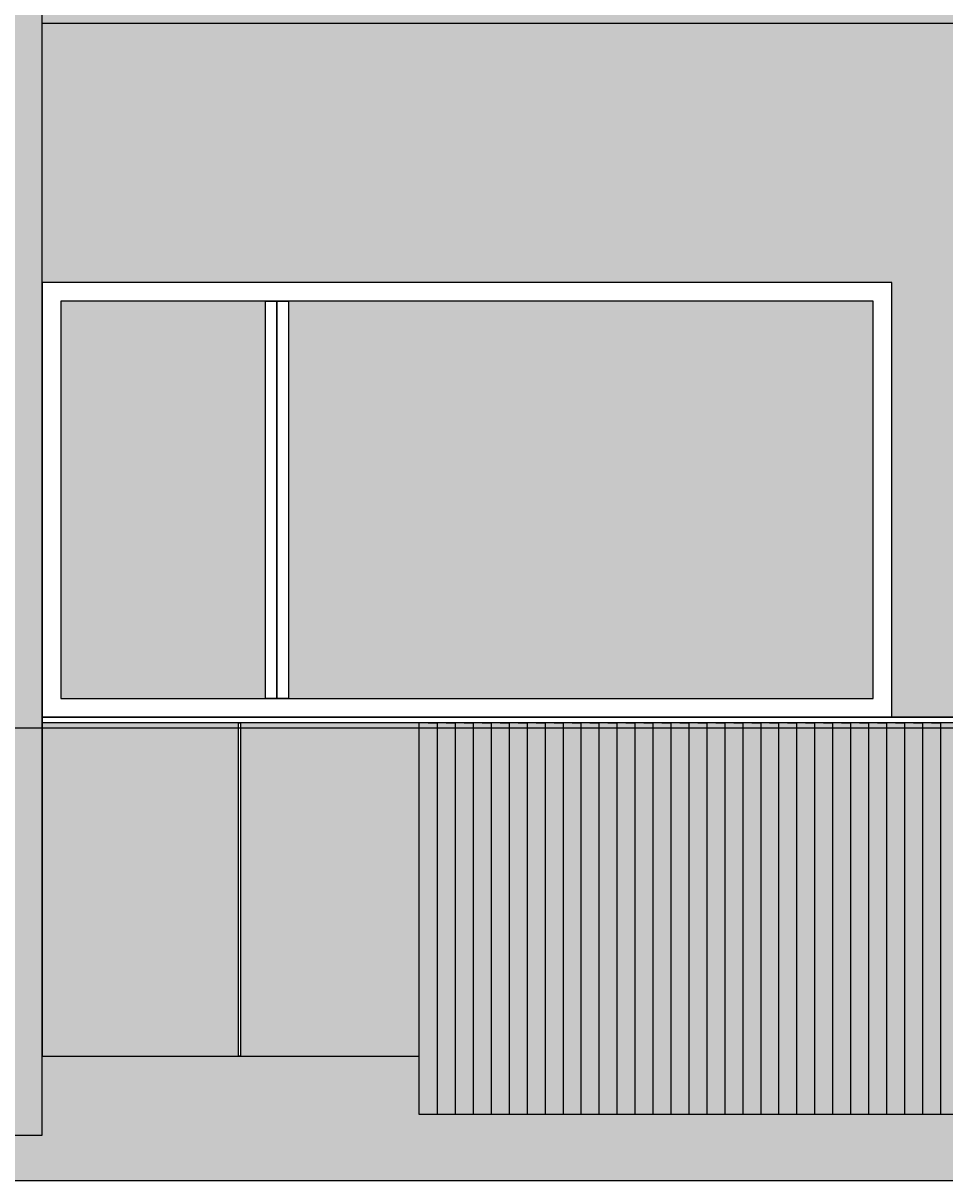
# Model space of a CAD drawing. Units: feet. Extents: x 2193 to 3502, y 890 to 1601.
# Tile 4 of 17: x 2466 to 2587, y 1073 to 1225. Entities that reach past the tile are written whole.
import ezdxf

# ---------------------------------------------------------------- set-up
doc = ezdxf.new("R2010")
doc.units = ezdxf.units.FT
for name, color, linetype, lineweight in [('A-ANNO-DIMS', 2, 'Continuous', 18), ('A-ELEV', 7, 'Continuous', 25), ('A-ELEV-PATT', 8, 'Continuous', 13)]:
    doc.layers.add(name, color=color, linetype=linetype, lineweight=lineweight)
doc.styles.get("Standard").update_dxf_attribs({"font": 'arial.ttf'})
doc.dimstyles.get("Standard").update_dxf_attribs({"dimtxt": 0.18, "dimasz": 0.18, "dimexe": 0.18, "dimexo": 0.0625, "dimgap": 0.09, "dimtad": 0, "dimtih": 1, "dimtoh": 1, "dimdec": 0, "dimzin": 0, "dimdsep": 46, "dimlunit": 3, "dimtxsty": 'Standard', "dimcen": 0.09, "dimadec": 0, "dimazin": 0, "dimtfac": 1, "dimtdec": 0, "dimtofl": 0, "dimtmove": 0, "dimatfit": 3, "dimfxl": 1, "dimtolj": 1, "dimtzin": 0, "dimarcsym": 0})

# ---------------------------------------------------------------- blocks, each defined once
blk = doc.blocks.new('*D19')
at = {"layer": 'A-ANNO-DIMS', "color": 0, "lineweight": -2, "transparency": 16777216}
for p, q in [((2934.31, 1073.03), (2193.56, 1073.03)), ((2193.74, 1072.85), (2193.74, 1012.11)), ((2193.74, 951), (2193.74, 1011.75)), ((2934.31, 950.82), (2193.56, 950.82))]:
    blk.add_line(p, q, dxfattribs=at)
at = {"layer": 'A-ANNO-DIMS', "color": 0, "transparency": 16777216}
for points in [[(2193.71, 1072.85), (2193.77, 1072.85), (2193.74, 1073.03)], [(2193.71, 951), (2193.77, 951), (2193.74, 950.82)]]:
    blk.add_solid(points, dxfattribs=at)
at = {"layer": 'Defpoints', "color": 0, "transparency": 16777216}
for p in [(2193.74, 1073.03), (2934.37, 1073.03), (2934.37, 950.82)]:
    blk.add_point(p, dxfattribs=at)
at = {"layer": 'A-ANNO-DIMS', "color": 0, "transparency": 16777216, "insert": (2193.74, 1011.93), "char_height": 0.18, "attachment_point": 5}
blk.add_mtext('\\A1;122.2', dxfattribs=at)
blk = doc.blocks.new('*D20')
at = {"layer": 'A-ANNO-DIMS', "color": 0, "lineweight": -2, "transparency": 16777216}
for p, q in [((2933.15, 1408.48), (2193.56, 1408.48)), ((2193.74, 1408.3), (2193.74, 1240.94)), ((2193.74, 1073.21), (2193.74, 1240.57)), ((2934.31, 1073.03), (2193.56, 1073.03))]:
    blk.add_line(p, q, dxfattribs=at)
at = {"layer": 'A-ANNO-DIMS', "color": 0, "transparency": 16777216}
for points in [[(2193.71, 1408.3), (2193.77, 1408.3), (2193.74, 1408.48)], [(2193.71, 1073.21), (2193.77, 1073.21), (2193.74, 1073.03)]]:
    blk.add_solid(points, dxfattribs=at)
at = {"layer": 'Defpoints', "color": 0, "transparency": 16777216}
for p in [(2193.74, 1408.48), (2933.21, 1408.48), (2934.37, 1073.03)]:
    blk.add_point(p, dxfattribs=at)
at = {"layer": 'A-ANNO-DIMS', "color": 0, "transparency": 16777216, "insert": (2193.74, 1240.76), "char_height": 0.18, "attachment_point": 5}
blk.add_mtext('\\A1;335.45', dxfattribs=at)
blk = doc.blocks.new('*D26')
at = {"layer": 'A-ANNO-DIMS', "color": 0, "lineweight": -2, "transparency": 16777216}
for p, q in [((2255.16, 950.89), (2255.16, 1601.47)), ((2255.34, 1601.29), (2507.42, 1601.29)), ((2760.29, 1601.29), (2508.21, 1601.29)), ((2760.47, 1541.11), (2760.47, 1601.47))]:
    blk.add_line(p, q, dxfattribs=at)
at = {"layer": 'A-ANNO-DIMS', "color": 0, "transparency": 16777216}
for points in [[(2255.34, 1601.32), (2255.34, 1601.26), (2255.16, 1601.29)], [(2760.29, 1601.32), (2760.29, 1601.26), (2760.47, 1601.29)]]:
    blk.add_solid(points, dxfattribs=at)
at = {"layer": 'Defpoints', "color": 0, "transparency": 16777216}
for p in [(2760.47, 1601.29), (2760.47, 1541.04), (2255.16, 950.82)]:
    blk.add_point(p, dxfattribs=at)
at = {"layer": 'A-ANNO-DIMS', "color": 0, "transparency": 16777216, "insert": (2507.82, 1601.29), "char_height": 0.18, "attachment_point": 5}
blk.add_mtext('\\A1;505.3', dxfattribs=at)
blk = doc.blocks.new('*D35')
at = {"layer": 'A-ANNO-DIMS', "color": 0, "lineweight": -2, "transparency": 16777216}
for p, q in [((2980.65, 1132.39), (2193.56, 1132.39)), ((2193.74, 1132.21), (2193.74, 1102.89)), ((2193.74, 1073.21), (2193.74, 1102.53)), ((2934.31, 1073.03), (2193.56, 1073.03))]:
    blk.add_line(p, q, dxfattribs=at)
at = {"layer": 'A-ANNO-DIMS', "color": 0, "transparency": 16777216}
for points in [[(2193.71, 1132.21), (2193.77, 1132.21), (2193.74, 1132.39)], [(2193.71, 1073.21), (2193.77, 1073.21), (2193.74, 1073.03)]]:
    blk.add_solid(points, dxfattribs=at)
at = {"layer": 'Defpoints', "color": 0, "transparency": 16777216}
for p in [(2193.74, 1132.39), (2980.72, 1132.39), (2934.37, 1073.03)]:
    blk.add_point(p, dxfattribs=at)
at = {"layer": 'A-ANNO-DIMS', "color": 0, "transparency": 16777216, "insert": (2193.74, 1102.71), "char_height": 0.18, "attachment_point": 5}
blk.add_mtext('\\A1;59.36', dxfattribs=at)
blk = doc.blocks.new('*D36')
at = {"layer": 'A-ANNO-DIMS', "color": 0, "lineweight": -2, "transparency": 16777216}
for p, q in [((2974.05, 1268.66), (2193.56, 1268.66)), ((2193.74, 1268.48), (2193.74, 1200.71)), ((2193.74, 1132.57), (2193.74, 1200.34)), ((2980.65, 1132.39), (2193.56, 1132.39))]:
    blk.add_line(p, q, dxfattribs=at)
at = {"layer": 'A-ANNO-DIMS', "color": 0, "transparency": 16777216}
for points in [[(2193.71, 1268.48), (2193.77, 1268.48), (2193.74, 1268.66)], [(2193.71, 1132.57), (2193.77, 1132.57), (2193.74, 1132.39)]]:
    blk.add_solid(points, dxfattribs=at)
at = {"layer": 'Defpoints', "color": 0, "transparency": 16777216}
for p in [(2193.74, 1268.66), (2974.12, 1268.66), (2980.72, 1132.39)]:
    blk.add_point(p, dxfattribs=at)
at = {"layer": 'A-ANNO-DIMS', "color": 0, "transparency": 16777216, "insert": (2193.74, 1200.53), "char_height": 0.18, "attachment_point": 5}
blk.add_mtext('\\A1;136.27', dxfattribs=at)

msp = doc.modelspace()

# ---------------------------------------------------------------- hatches: boundary and pattern name
at = {"layer": 'A-ELEV-PATT'}
h = msp.add_hatch(color=256, dxfattribs=at)
h.dxf.hatch_style = 1
h.paths.add_polyline_path([(2760.4733, 1512.3957), (2586.1736, 1512.3957), (2586.1736, 1502.0763), (2602.8648, 1502.0763), (2699.5726, 1502.0763), (2699.6322, 1502.0763), (2760.4733, 1502.0763)])
h.paths.add_polyline_path([(2760.4733, 1382.0763), (2275.0482, 1382.0763), (2275.0482, 1367.5739), (2745.971, 1367.5739), (2745.971, 1166.2327), (2760.4733, 1166.2327)])
h.paths.add_polyline_path([(2468.2854, 1266.7092), (2294.8992, 1266.7092), (2294.8992, 1079.031), (2468.2854, 1079.031)])
h.paths.add_polyline_path([(2301.4984, 1260.11), (2461.6863, 1260.11), (2461.6863, 1085.6301), (2301.4984, 1085.6301)], flags=16)
h.paths.add_polyline_path([(2452.7821, 1241.1967), (2452.7821, 1217.2819), (2454.6216, 1217.2819), (2454.6216, 1133.1367), (2461.6863, 1133.1367), (2461.6863, 1132.3937), (2381.7172, 1132.3937), (2381.7172, 1085.6301), (2381.4675, 1085.6301), (2381.4675, 1132.3937), (2301.4984, 1132.3937), (2301.4984, 1133.1367), (2301.4984, 1217.2819), (2390.8933, 1217.2819), (2390.8933, 1241.1967)], flags=0)
h.paths.add_polyline_path([(2372.4936, 1214.8367), (2372.4936, 1133.1367), (2371.1246, 1133.1367), (2371.1246, 1214.8367), (2337.2323, 1214.8367), (2337.2323, 1133.1367), (2335.8632, 1133.1367), (2335.8632, 1214.8367), (2337.2323, 1214.8367)], flags=0)
h = msp.add_hatch(color=256, dxfattribs=at)
h.dxf.hatch_style = 1
h.paths.add_polyline_path([(2576.3428, 1407.7384), (2536.5416, 1407.7384), (2536.5416, 1406.15), (2536.5416, 1382.0763), (2576.3428, 1382.0763)])
h.paths.add_polyline_path([(2627.3548, 1407.7384), (2576.5924, 1407.7384), (2576.5924, 1382.0763), (2627.3548, 1382.0763)])
h.paths.add_polyline_path([(2667.9236, 1407.7384), (2627.6045, 1407.7384), (2627.6045, 1382.0763), (2667.9236, 1382.0763)])
h.paths.add_polyline_path([(2699.6322, 1407.7384), (2668.1733, 1407.7384), (2668.1733, 1382.0763), (2699.6322, 1382.0763)])
h.paths.add_polyline_path([(2497.5717, 1323.2248), (2470.7305, 1323.2248), (2470.7305, 1271.105), (2497.5717, 1271.105)])
h.paths.add_polyline_path([(2577.3219, 1323.2248), (2500.599, 1323.2248), (2500.599, 1271.105), (2577.3219, 1271.105)])
h.paths.add_polyline_path([(2388.4482, 1327.1314), (2343.4244, 1327.1314), (2343.4244, 1268.6599), (2388.4482, 1268.6599)])
h.paths.add_polyline_path([(2342.3682, 1327.1314), (2297.3443, 1327.1314), (2297.3443, 1268.6599), (2342.3682, 1268.6599)])
h.paths.add_polyline_path([(2335.8632, 1214.8367), (2301.4984, 1214.8367), (2301.4984, 1133.1367), (2335.8632, 1133.1367)])
h.paths.add_polyline_path([(2371.1246, 1214.8367), (2337.2323, 1214.8367), (2337.2323, 1133.1367), (2371.1246, 1133.1367)])
h.paths.add_polyline_path([(2390.8933, 1214.8367), (2372.4936, 1214.8367), (2372.4936, 1133.1367), (2390.8933, 1133.1367)])
h.paths.add_polyline_path([(2577.3219, 1188.4208), (2500.599, 1188.4208), (2500.599, 1136.3009), (2577.3219, 1136.3009)])
h.paths.add_polyline_path([(2497.5717, 1188.4208), (2470.7305, 1188.4208), (2470.7305, 1136.3009), (2497.5717, 1136.3009)])
h.paths.add_polyline_path([(2381.4675, 1132.3937), (2301.4984, 1132.3937), (2301.4984, 1085.6301), (2381.4675, 1085.6301)])
h.paths.add_polyline_path([(2461.6863, 1132.3937), (2381.7172, 1132.3937), (2381.7172, 1085.6301), (2461.6863, 1085.6301)])
h.paths.add_polyline_path([(2494.0463, 1133.1128), (2468.2854, 1133.1128), (2468.2854, 1089.3627), (2494.0463, 1089.3627)])
h.paths.add_polyline_path([(2517.7591, 1133.1128), (2494.296, 1133.1128), (2494.296, 1089.3627), (2517.7591, 1089.3627)])
h.paths.add_polyline_path([(2667.9236, 1133.1128), (2636.5184, 1133.1128), (2636.5184, 1089.3627), (2667.9236, 1089.3627)])
h.paths.add_polyline_path([(2699.6322, 1133.1128), (2668.1733, 1133.1128), (2668.1733, 1089.3627), (2699.6322, 1089.3627)])
h.paths.add_polyline_path([(2651.839, 1070.5859), (2638.7977, 1070.5859), (2638.7977, 1047.0961), (2651.839, 1047.0961)])
h.paths.add_polyline_path([(2637.6317, 1070.5859), (2625.7563, 1070.5859), (2625.7563, 1047.0961), (2637.6317, 1047.0961)])
h.paths.add_polyline_path([(2583.4393, 1052.8618), (2515.9216, 1052.8618), (2515.9216, 1032.1935), (2583.4393, 1032.1935)])
h.paths.add_polyline_path([(2514.4293, 1052.8618), (2492.062, 1052.8618), (2492.062, 1032.1935), (2514.4293, 1032.1935)])
h.paths.add_polyline_path([(2388.4482, 1038.8658), (2348.7682, 1038.8658), (2348.7682, 988.9597), (2388.4482, 988.9597)])
h.paths.add_polyline_path([(2346.3231, 1038.8658), (2309.0883, 1038.8658), (2309.0883, 988.9597), (2346.3231, 988.9597)])
h.paths.add_polyline_path([(2667.9236, 1267.9169), (2636.5184, 1267.9169), (2636.5184, 1241.1967), (2667.9236, 1241.1967)])
h.paths.add_polyline_path([(2699.6322, 1267.9169), (2668.1733, 1267.9169), (2668.1733, 1241.1967), (2699.6322, 1241.1967)])
h.paths.add_polyline_path([(2517.7591, 1267.9169), (2494.296, 1267.9169), (2494.296, 1241.1967), (2517.7591, 1241.1967)])
h.paths.add_polyline_path([(2494.0463, 1267.9169), (2468.2854, 1267.9169), (2468.2854, 1266.7092), (2468.2854, 1241.1967), (2494.0463, 1241.1967)])
h = msp.add_hatch(color=256, dxfattribs=at)
h.dxf.hatch_style = 1
h.paths.add_polyline_path([(2294.8992, 1367.5739), (2275.0482, 1367.5739), (2275.0482, 1382.0763), (2536.5416, 1382.0763), (2536.5416, 1406.15), (2256.3232, 1406.15), (2256.3232, 1089.3627), (2255.1574, 1089.3627), (2255.1574, 1073.031), (2294.8992, 1073.031)])
h.paths.add_polyline_path([(2517.7591, 1241.1967), (2468.2854, 1241.1967), (2468.2854, 1224.865), (2598.591, 1224.865), (2598.591, 1233.561), (2517.7591, 1233.561)])
h.paths.add_polyline_path([(2699.6322, 1241.1967), (2636.5184, 1241.1967), (2636.5184, 1233.561), (2616.5596, 1233.561), (2616.5596, 1224.865), (2699.6322, 1224.865)])
h.paths.add_polyline_path([(2615.4622, 1233.561), (2613.8564, 1233.561), (2613.8564, 1224.865), (2615.4622, 1224.865)])
h.paths.add_polyline_path([(2612.759, 1233.561), (2609.5836, 1233.561), (2609.5836, 1224.865), (2612.759, 1224.865)])
h.paths.add_polyline_path([(2608.4862, 1233.561), (2606.5316, 1233.561), (2606.5316, 1224.865), (2608.4862, 1224.865)])
h.paths.add_polyline_path([(2605.4342, 1233.561), (2602.5204, 1233.561), (2602.5204, 1224.865), (2605.4342, 1224.865)])
h.paths.add_polyline_path([(2601.423, 1233.561), (2599.6883, 1233.561), (2599.6883, 1224.865), (2601.423, 1224.865)])
h.paths.add_polyline_path([(2517.7591, 1089.3627), (2468.2854, 1089.3627), (2468.2854, 1079.031), (2294.8992, 1079.031), (2294.8992, 1073.031), (2390.8933, 1073.031), (2452.7821, 1073.031), (2760.4733, 1073.031), (2760.4733, 1089.3627), (2699.6322, 1089.3627), (2636.5184, 1089.3627), (2636.5184, 1081.7269), (2517.7591, 1081.7269)])
h = msp.add_hatch(color=256, dxfattribs=at)
h.dxf.hatch_style = 1
h.paths.add_polyline_path([(2452.7821, 1355.2199), (2622.9814, 1355.2199), (2622.9814, 1268.6599), (2646.2844, 1268.6599), (2646.2844, 1367.5739), (2390.8933, 1367.5739), (2390.8933, 1268.6599), (2452.7821, 1268.6599)])
h.paths.add_polyline_path([(2452.7821, 1016.4), (2431.9134, 1016.4), (2431.9134, 1032.1935), (2452.7821, 1032.1935), (2452.7821, 1073.031), (2390.8933, 1073.031), (2390.8933, 956.8829), (2452.7821, 956.8829)])
h.paths.add_polyline_path([(2452.7821, 1241.1967), (2390.8933, 1241.1967), (2390.8933, 1133.1367), (2452.7821, 1133.1367)])
h.paths.add_polyline_path([(2636.5184, 1267.9169), (2517.7591, 1267.9169), (2517.7591, 1233.561), (2598.591, 1233.561), (2598.591, 1249.8256), (2599.6883, 1249.8256), (2599.6883, 1233.561), (2601.423, 1233.561), (2601.423, 1247.0422), (2602.5204, 1247.0422), (2602.5204, 1233.561), (2605.4342, 1233.561), (2605.4342, 1250.4403), (2606.5316, 1250.4403), (2606.5316, 1233.561), (2608.4862, 1233.561), (2608.4862, 1248.4363), (2609.5836, 1248.4363), (2609.5836, 1233.561), (2612.759, 1233.561), (2612.759, 1243.2956), (2613.8564, 1243.2956), (2613.8564, 1233.561), (2615.4622, 1233.561), (2615.4622, 1249.6561), (2616.5596, 1249.6561), (2616.5596, 1233.561), (2636.5184, 1233.561)])
h.paths.add_polyline_path([(2601.423, 1133.1128), (2599.6883, 1133.1128), (2599.6883, 1115.2331), (2598.591, 1115.2331), (2598.591, 1133.1128), (2517.7591, 1133.1128), (2517.7591, 1081.7269), (2636.5184, 1081.7269), (2636.5184, 1133.1128), (2616.5596, 1133.1128), (2616.5596, 1115.0637), (2615.4622, 1115.0637), (2615.4622, 1133.1128), (2613.8564, 1133.1128), (2613.8564, 1108.7032), (2612.759, 1108.7032), (2612.759, 1133.1128), (2609.5836, 1133.1128), (2609.5836, 1113.8439), (2608.4862, 1113.8439), (2608.4862, 1133.1128), (2606.5316, 1133.1128), (2606.5316, 1115.8479), (2605.4342, 1115.8479), (2605.4342, 1133.1128), (2602.5204, 1133.1128), (2602.5204, 1112.4498), (2601.423, 1112.4498)])
h = msp.add_hatch(color=256, dxfattribs=at)
h.dxf.hatch_style = 1
h.paths.add_polyline_path([(2622.9814, 1355.2199), (2452.7821, 1355.2199), (2452.7821, 1268.6599), (2468.2854, 1268.6599), (2468.2854, 1325.6699), (2579.767, 1325.6699), (2579.767, 1268.6599), (2622.9814, 1268.6599)])
h.paths.add_polyline_path([(2598.591, 1224.865), (2468.2854, 1224.865), (2468.2854, 1190.8659), (2579.767, 1190.8659), (2579.767, 1133.8558), (2598.591, 1133.8558)])
h.paths.add_polyline_path([(2390.8933, 1241.1967), (2301.4984, 1241.1967), (2301.4984, 1224.865), (2390.8933, 1224.865)])
h.paths.add_polyline_path([(3070.1101, 1073.031), (2940.0814, 1073.031), (2940.0814, 956.5285), (2940.6598, 956.8829), (3070.1101, 956.8829), (3070.1101, 986.5146), (2985.8599, 986.5146), (2985.8599, 1041.3109), (3070.1101, 1041.3109)])

# ---------------------------------------------------------------- linework, layer by layer
at = {"layer": 'A-ELEV'}
for p, q in [((2468.2854, 1224.865), (2699.6322, 1224.865)), ((2468.2854, 1089.3627), (2517.7591, 1089.3627)), ((2468.2854, 1089.3627), (2517.7591, 1089.3627))]:
    msp.add_line(p, q, dxfattribs=at)
for points in [[(2294.8992, 1079.031), (2468.2854, 1079.031), (2468.2854, 1266.7092), (2294.8992, 1266.7092)], [(2294.8992, 1079.031), (2468.2854, 1079.031), (2468.2854, 1266.7092), (2294.8992, 1266.7092)], [(2468.2854, 1133.8558), (2579.767, 1133.8558), (2579.767, 1190.8659), (2468.2854, 1190.8659)], [(2468.2854, 1133.8558), (2579.767, 1133.8558), (2579.767, 1190.8659), (2468.2854, 1190.8659)], [(2470.7305, 1136.3009), (2577.3219, 1136.3009), (2577.3219, 1188.4208), (2470.7305, 1188.4208)], [(2470.7305, 1136.3009), (2577.3219, 1136.3009), (2577.3219, 1188.4208), (2470.7305, 1188.4208)], [(2497.5717, 1188.4208), (2499.0853, 1188.4208), (2499.0853, 1136.3009), (2497.5717, 1136.3009)], [(2497.5717, 1188.4208), (2499.0853, 1188.4208), (2499.0853, 1136.3009), (2497.5717, 1136.3009)], [(2499.0853, 1188.4208), (2500.599, 1188.4208), (2500.599, 1136.3009), (2499.0853, 1136.3009)], [(2499.0853, 1188.4208), (2500.599, 1188.4208), (2500.599, 1136.3009), (2499.0853, 1136.3009)], [(2494.0463, 1133.1128), (2494.296, 1133.1128), (2494.296, 1089.3627), (2494.0463, 1089.3627)], [(2494.0463, 1133.1128), (2494.296, 1133.1128), (2494.296, 1089.3627), (2494.0463, 1089.3627)]]:
    msp.add_lwpolyline(points, close=True, dxfattribs=at)
for points in [[(2699.6322, 1133.8558), (2468.2854, 1133.8558), (2468.2854, 1089.3627)], [(2699.6322, 1133.1128), (2468.2854, 1133.1128), (2468.2854, 1133.8558), (2699.6322, 1133.8558)], [(2598.591, 1133.8558), (2468.2854, 1133.8558), (2468.2854, 1089.3627)], [(2598.591, 1133.1128), (2468.2854, 1133.1128), (2468.2854, 1133.8558), (2598.591, 1133.8558)], [(2636.5184, 1133.1128), (2636.5184, 1081.7269), (2517.7591, 1081.7269), (2517.7591, 1133.1128)], [(2636.5184, 1133.1128), (2636.5184, 1081.7269), (2517.7591, 1081.7269), (2517.7591, 1133.1128)], [(2518.938, 1133.1128), (2520.1169, 1133.1128), (2520.1169, 1081.7269), (2518.938, 1081.7269)], [(2521.2958, 1133.1128), (2522.4747, 1133.1128), (2522.4747, 1081.7269), (2521.2958, 1081.7269)], [(2523.6536, 1133.1128), (2524.8326, 1133.1128), (2524.8326, 1081.7269), (2523.6536, 1081.7269)], [(2526.0115, 1133.1128), (2527.1904, 1133.1128), (2527.1904, 1081.7269), (2526.0115, 1081.7269)], [(2528.3693, 1133.1128), (2529.5482, 1133.1128), (2529.5482, 1081.7269), (2528.3693, 1081.7269)], [(2530.7272, 1133.1128), (2531.9061, 1133.1128), (2531.9061, 1081.7269), (2530.7272, 1081.7269)], [(2533.085, 1133.1128), (2534.2639, 1133.1128), (2534.2639, 1081.7269), (2533.085, 1081.7269)], [(2535.4428, 1133.1128), (2536.6217, 1133.1128), (2536.6217, 1081.7269), (2535.4428, 1081.7269)], [(2537.8007, 1133.1128), (2538.9796, 1133.1128), (2538.9796, 1081.7269), (2537.8007, 1081.7269)], [(2540.1585, 1133.1128), (2541.3374, 1133.1128), (2541.3374, 1081.7269), (2540.1585, 1081.7269)], [(2542.5163, 1133.1128), (2543.6953, 1133.1128), (2543.6953, 1081.7269), (2542.5163, 1081.7269)], [(2544.8742, 1133.1128), (2546.0531, 1133.1128), (2546.0531, 1081.7269), (2544.8742, 1081.7269)], [(2547.232, 1133.1128), (2548.4109, 1133.1128), (2548.4109, 1081.7269), (2547.232, 1081.7269)], [(2549.5899, 1133.1128), (2550.7688, 1133.1128), (2550.7688, 1081.7269), (2549.5899, 1081.7269)], [(2551.9477, 1133.1128), (2553.1266, 1133.1128), (2553.1266, 1081.7269), (2551.9477, 1081.7269)], [(2554.3055, 1133.1128), (2555.4844, 1133.1128), (2555.4844, 1081.7269), (2554.3055, 1081.7269)], [(2556.6634, 1133.1128), (2557.8423, 1133.1128), (2557.8423, 1081.7269), (2556.6634, 1081.7269)], [(2559.0212, 1133.1128), (2560.2001, 1133.1128), (2560.2001, 1081.7269), (2559.0212, 1081.7269)], [(2561.379, 1133.1128), (2562.558, 1133.1128), (2562.558, 1081.7269), (2561.379, 1081.7269)], [(2563.7369, 1133.1128), (2564.9158, 1133.1128), (2564.9158, 1081.7269), (2563.7369, 1081.7269)], [(2566.0947, 1133.1128), (2567.2736, 1133.1128), (2567.2736, 1081.7269), (2566.0947, 1081.7269)], [(2568.4525, 1133.1128), (2569.6315, 1133.1128), (2569.6315, 1081.7269), (2568.4525, 1081.7269)], [(2570.8104, 1133.1128), (2571.9893, 1133.1128), (2571.9893, 1081.7269), (2570.8104, 1081.7269)], [(2573.1682, 1133.1128), (2574.3471, 1133.1128), (2574.3471, 1081.7269), (2573.1682, 1081.7269)], [(2575.5261, 1133.1128), (2576.705, 1133.1128), (2576.705, 1081.7269), (2575.5261, 1081.7269)], [(2577.8839, 1133.1128), (2579.0628, 1133.1128), (2579.0628, 1081.7269), (2577.8839, 1081.7269)], [(2580.2417, 1133.1128), (2581.4207, 1133.1128), (2581.4207, 1081.7269), (2580.2417, 1081.7269)], [(2582.5996, 1133.1128), (2583.7785, 1133.1128), (2583.7785, 1081.7269), (2582.5996, 1081.7269)], [(2584.9574, 1133.1128), (2586.1363, 1133.1128), (2586.1363, 1081.7269), (2584.9574, 1081.7269)]]:
    msp.add_lwpolyline(points, dxfattribs=at)

# ---------------------------------------------------------------- dimensions: what is measured, and where the dimension line sits
at = {"layer": 'A-ANNO-DIMS'}
dim = msp.add_linear_dim(base=(2760.4733, 1601.2941), p1=(2255.1574, 950.8228), p2=(2760.4733, 1541.0441), dimstyle='Standard', override={"dimdec": 1, "dimlfac": 1, "dimrnd": 0, "dimzin": 0, "dimdsep": 46, "dimlunit": 2}, dxfattribs=at)
dim.commit()
dim.dimension.update_dxf_attribs({"geometry": '*D26', "text_midpoint": (2507.8154, 1601.2941)})
for base, p1, p2, override, picture, middle in [((2193.7417, 1408.4814), (2934.3742, 1073.031), (2933.2085, 1408.4814), {"dimdec": 2, "dimlfac": 1, "dimrnd": 0, "dimzin": 0, "dimdsep": 46, "dimlunit": 2}, '*D20', (2193.7417, 1240.7562)), ((2193.7417, 1268.6599), (2980.7151, 1132.3937), (2974.116, 1268.6599), {"dimdec": 2, "dimlfac": 1, "dimrnd": 0, "dimzin": 0, "dimdsep": 46, "dimlunit": 2}, '*D36', (2193.7417, 1200.5268)), ((2193.7417, 1132.3937), (2934.3742, 1073.031), (2980.7151, 1132.3937), {"dimdec": 2, "dimlfac": 1, "dimrnd": 0, "dimzin": 0, "dimdsep": 46, "dimlunit": 2}, '*D35', (2193.7417, 1102.7124)), ((2193.7417, 1073.031), (2934.3742, 950.8228), (2934.3742, 1073.031), {"dimdec": 1, "dimlfac": 1, "dimrnd": 0, "dimzin": 0, "dimdsep": 46, "dimlunit": 2}, '*D19', (2193.7417, 1011.9269))]:
    dim = msp.add_linear_dim(base=base, p1=p1, p2=p2, angle=90, dimstyle='Standard', override=override, dxfattribs=at)
    dim.commit()
    dim.dimension.update_dxf_attribs({"geometry": picture, "text_midpoint": middle})

doc.saveas('drawing.dxf')
